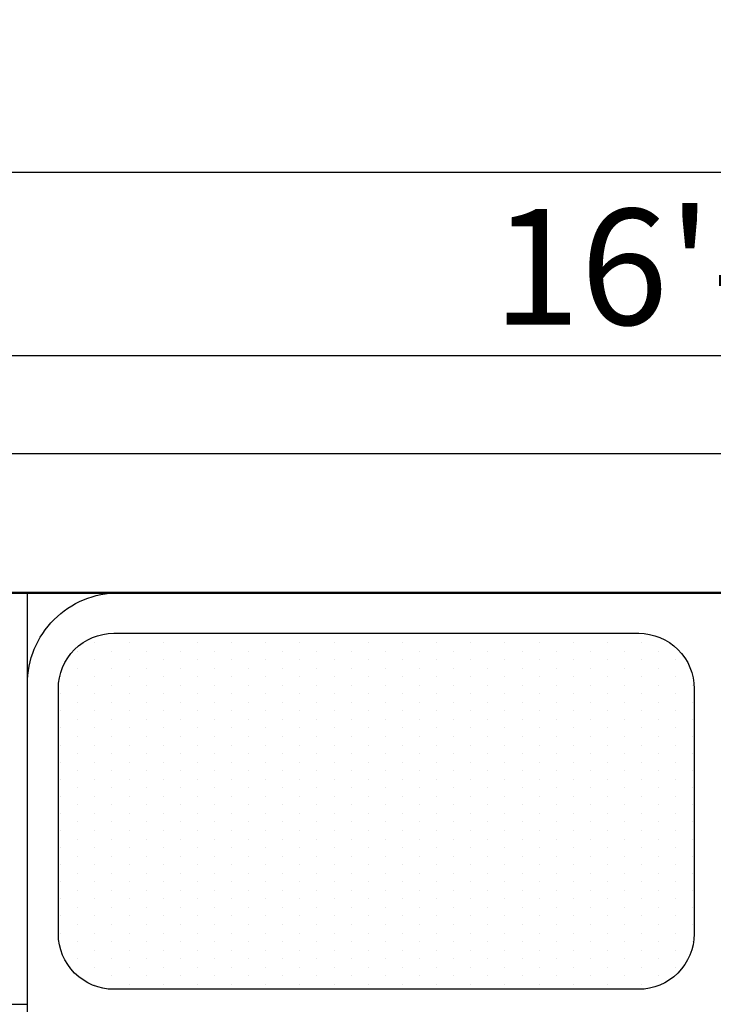
# Model space of a CAD drawing. Units: inches. Extents: x 3064 to 19385, y 846 to 15425.
# Tile 62 of 108: x 6251 to 6281, y 1964 to 2007. Entities that reach past the tile are written whole.
import ezdxf

# ---------------------------------------------------------------- set-up
doc = ezdxf.new("R2010")
doc.units = ezdxf.units.IN
for name, color, linetype, lineweight in [('A-ANNO-DIMS', 2, 'Continuous', 18), ('A-FLOR-FIXT', 9, 'Continuous', 18), ('A-WALL', 7, 'Continuous', 50), ('C-PROP', 6, 'Continuous', 25)]:
    doc.layers.add(name, color=color, linetype=linetype, lineweight=lineweight)
doc.layers.add('BLOCK', color=6, linetype='Continuous')
doc.styles.get("Standard").update_dxf_attribs({"font": 'arial.ttf'})
doc.dimstyles.new('ISO-25', dxfattribs={"dimtxt": 9, "dimasz": 2.5, "dimexe": 1.25, "dimexo": 0.625, "dimtad": 1, "dimdec": 1, "dimlunit": 3, "dimtxsty": 'Standard', "dimcen": 2.5, "dimadec": 0, "dimazin": 0, "dimtfac": 1, "dimtdec": 1, "dimtmove": 0, "dimatfit": 3, "dimfxl": 1, "dimarcsym": 0})

# ---------------------------------------------------------------- blocks, each defined once
blk = doc.blocks.new('*X7')
at = {"color": 0}
for p, q in [((266.25, 456.9375), (266.25, 456.9375)), ((266.4375, 457.03125), (266.4375, 457.03125)), ((266.625, 456.9375), (266.625, 456.9375)), ((266.8125, 457.03125), (266.8125, 457.03125)), ((267, 456.9375), (267, 456.9375)), ((267.1875, 457.03125), (267.1875, 457.03125)), ((267.375, 456.9375), (267.375, 456.9375)), ((267.5625, 457.03125), (267.5625, 457.03125)), ((267.75, 456.9375), (267.75, 456.9375)), ((267.9375, 457.03125), (267.9375, 457.03125)), ((268.125, 456.9375), (268.125, 456.9375)), ((268.3125, 457.03125), (268.3125, 457.03125)), ((268.5, 456.9375), (268.5, 456.9375)), ((268.6875, 457.03125), (268.6875, 457.03125)), ((268.875, 456.9375), (268.875, 456.9375)), ((269.0625, 457.03125), (269.0625, 457.03125)), ((269.25, 456.9375), (269.25, 456.9375)), ((269.4375, 457.03125), (269.4375, 457.03125)), ((269.625, 456.9375), (269.625, 456.9375)), ((269.8125, 457.03125), (269.8125, 457.03125)), ((270, 456.9375), (270, 456.9375)), ((270.1875, 457.03125), (270.1875, 457.03125)), ((270.375, 456.9375), (270.375, 456.9375)), ((270.5625, 457.03125), (270.5625, 457.03125)), ((270.75, 456.9375), (270.75, 456.9375)), ((270.9375, 457.03125), (270.9375, 457.03125)), ((271.125, 456.9375), (271.125, 456.9375)), ((271.3125, 457.03125), (271.3125, 457.03125)), ((271.5, 456.9375), (271.5, 456.9375)), ((271.6875, 457.03125), (271.6875, 457.03125)), ((271.875, 456.9375), (271.875, 456.9375)), ((272.0625, 457.03125), (272.0625, 457.03125)), ((272.25, 456.9375), (272.25, 456.9375)), ((266.0625, 456.84375), (266.0625, 456.84375)), ((266.4375, 456.84375), (266.4375, 456.84375)), ((266.8125, 456.84375), (266.8125, 456.84375)), ((267.1875, 456.84375), (267.1875, 456.84375)), ((267.5625, 456.84375), (267.5625, 456.84375)), ((267.9375, 456.84375), (267.9375, 456.84375)), ((268.3125, 456.84375), (268.3125, 456.84375)), ((268.6875, 456.84375), (268.6875, 456.84375)), ((269.0625, 456.84375), (269.0625, 456.84375)), ((269.4375, 456.84375), (269.4375, 456.84375)), ((269.8125, 456.84375), (269.8125, 456.84375)), ((270.1875, 456.84375), (270.1875, 456.84375)), ((270.5625, 456.84375), (270.5625, 456.84375)), ((270.9375, 456.84375), (270.9375, 456.84375)), ((271.3125, 456.84375), (271.3125, 456.84375)), ((271.6875, 456.84375), (271.6875, 456.84375)), ((272.0625, 456.84375), (272.0625, 456.84375)), ((272.4375, 456.84375), (272.4375, 456.84375)), ((266.25, 456.75), (266.25, 456.75)), ((266.625, 456.75), (266.625, 456.75)), ((267, 456.75), (267, 456.75)), ((267.375, 456.75), (267.375, 456.75)), ((267.75, 456.75), (267.75, 456.75)), ((268.125, 456.75), (268.125, 456.75)), ((268.5, 456.75), (268.5, 456.75)), ((268.875, 456.75), (268.875, 456.75)), ((269.25, 456.75), (269.25, 456.75)), ((269.625, 456.75), (269.625, 456.75)), ((270, 456.75), (270, 456.75)), ((270.375, 456.75), (270.375, 456.75)), ((270.75, 456.75), (270.75, 456.75)), ((271.125, 456.75), (271.125, 456.75)), ((271.5, 456.75), (271.5, 456.75)), ((271.875, 456.75), (271.875, 456.75)), ((272.25, 456.75), (272.25, 456.75)), ((272.625, 456.75), (272.625, 456.75)), ((266.0625, 456.65625), (266.0625, 456.65625)), ((266.4375, 456.65625), (266.4375, 456.65625)), ((266.8125, 456.65625), (266.8125, 456.65625)), ((267.1875, 456.65625), (267.1875, 456.65625)), ((267.5625, 456.65625), (267.5625, 456.65625)), ((267.9375, 456.65625), (267.9375, 456.65625)), ((268.3125, 456.65625), (268.3125, 456.65625)), ((268.6875, 456.65625), (268.6875, 456.65625)), ((269.0625, 456.65625), (269.0625, 456.65625)), ((269.4375, 456.65625), (269.4375, 456.65625)), ((269.8125, 456.65625), (269.8125, 456.65625)), ((270.1875, 456.65625), (270.1875, 456.65625)), ((270.5625, 456.65625), (270.5625, 456.65625)), ((270.9375, 456.65625), (270.9375, 456.65625)), ((271.3125, 456.65625), (271.3125, 456.65625)), ((271.6875, 456.65625), (271.6875, 456.65625)), ((272.0625, 456.65625), (272.0625, 456.65625)), ((272.4375, 456.65625), (272.4375, 456.65625)), ((265.875, 456.5625), (265.875, 456.5625)), ((266.25, 456.5625), (266.25, 456.5625)), ((266.625, 456.5625), (266.625, 456.5625)), ((267, 456.5625), (267, 456.5625)), ((267.375, 456.5625), (267.375, 456.5625)), ((267.75, 456.5625), (267.75, 456.5625)), ((268.125, 456.5625), (268.125, 456.5625)), ((268.5, 456.5625), (268.5, 456.5625)), ((268.875, 456.5625), (268.875, 456.5625)), ((269.25, 456.5625), (269.25, 456.5625)), ((269.625, 456.5625), (269.625, 456.5625)), ((270, 456.5625), (270, 456.5625)), ((270.375, 456.5625), (270.375, 456.5625)), ((270.75, 456.5625), (270.75, 456.5625)), ((271.125, 456.5625), (271.125, 456.5625)), ((271.5, 456.5625), (271.5, 456.5625)), ((271.875, 456.5625), (271.875, 456.5625)), ((272.25, 456.5625), (272.25, 456.5625)), ((272.625, 456.5625), (272.625, 456.5625)), ((266.0625, 456.46875), (266.0625, 456.46875)), ((266.4375, 456.46875), (266.4375, 456.46875)), ((266.8125, 456.46875), (266.8125, 456.46875)), ((267.1875, 456.46875), (267.1875, 456.46875)), ((267.5625, 456.46875), (267.5625, 456.46875)), ((267.9375, 456.46875), (267.9375, 456.46875)), ((268.3125, 456.46875), (268.3125, 456.46875)), ((268.6875, 456.46875), (268.6875, 456.46875)), ((269.0625, 456.46875), (269.0625, 456.46875)), ((269.4375, 456.46875), (269.4375, 456.46875)), ((269.8125, 456.46875), (269.8125, 456.46875)), ((270.1875, 456.46875), (270.1875, 456.46875)), ((270.5625, 456.46875), (270.5625, 456.46875)), ((270.9375, 456.46875), (270.9375, 456.46875)), ((271.3125, 456.46875), (271.3125, 456.46875)), ((271.6875, 456.46875), (271.6875, 456.46875)), ((272.0625, 456.46875), (272.0625, 456.46875)), ((272.4375, 456.46875), (272.4375, 456.46875)), ((272.8125, 456.46875), (272.8125, 456.46875)), ((265.875, 456.375), (265.875, 456.375)), ((266.25, 456.375), (266.25, 456.375)), ((266.625, 456.375), (266.625, 456.375)), ((267, 456.375), (267, 456.375)), ((267.375, 456.375), (267.375, 456.375)), ((267.75, 456.375), (267.75, 456.375)), ((268.125, 456.375), (268.125, 456.375)), ((268.5, 456.375), (268.5, 456.375)), ((268.875, 456.375), (268.875, 456.375)), ((269.25, 456.375), (269.25, 456.375)), ((269.625, 456.375), (269.625, 456.375)), ((270, 456.375), (270, 456.375)), ((270.375, 456.375), (270.375, 456.375)), ((270.75, 456.375), (270.75, 456.375)), ((271.125, 456.375), (271.125, 456.375)), ((271.5, 456.375), (271.5, 456.375)), ((271.875, 456.375), (271.875, 456.375)), ((272.25, 456.375), (272.25, 456.375)), ((272.625, 456.375), (272.625, 456.375)), ((265.875, 456.1875), (265.875, 456.1875)), ((266.0625, 456.28125), (266.0625, 456.28125)), ((266.25, 456.1875), (266.25, 456.1875)), ((266.4375, 456.28125), (266.4375, 456.28125)), ((266.625, 456.1875), (266.625, 456.1875)), ((266.8125, 456.28125), (266.8125, 456.28125)), ((267, 456.1875), (267, 456.1875)), ((267.1875, 456.28125), (267.1875, 456.28125)), ((267.375, 456.1875), (267.375, 456.1875)), ((267.5625, 456.28125), (267.5625, 456.28125)), ((267.75, 456.1875), (267.75, 456.1875)), ((267.9375, 456.28125), (267.9375, 456.28125)), ((268.125, 456.1875), (268.125, 456.1875)), ((268.3125, 456.28125), (268.3125, 456.28125)), ((268.5, 456.1875), (268.5, 456.1875)), ((268.6875, 456.28125), (268.6875, 456.28125)), ((268.875, 456.1875), (268.875, 456.1875)), ((269.0625, 456.28125), (269.0625, 456.28125)), ((269.25, 456.1875), (269.25, 456.1875)), ((269.4375, 456.28125), (269.4375, 456.28125)), ((269.625, 456.1875), (269.625, 456.1875)), ((269.8125, 456.28125), (269.8125, 456.28125)), ((270, 456.1875), (270, 456.1875)), ((270.1875, 456.28125), (270.1875, 456.28125)), ((270.375, 456.1875), (270.375, 456.1875)), ((270.5625, 456.28125), (270.5625, 456.28125)), ((270.75, 456.1875), (270.75, 456.1875)), ((270.9375, 456.28125), (270.9375, 456.28125)), ((271.125, 456.1875), (271.125, 456.1875)), ((271.3125, 456.28125), (271.3125, 456.28125)), ((271.5, 456.1875), (271.5, 456.1875)), ((271.6875, 456.28125), (271.6875, 456.28125)), ((271.875, 456.1875), (271.875, 456.1875)), ((272.0625, 456.28125), (272.0625, 456.28125)), ((272.25, 456.1875), (272.25, 456.1875)), ((272.4375, 456.28125), (272.4375, 456.28125)), ((272.625, 456.1875), (272.625, 456.1875)), ((272.8125, 456.28125), (272.8125, 456.28125)), ((266.0625, 456.09375), (266.0625, 456.09375)), ((266.4375, 456.09375), (266.4375, 456.09375)), ((266.8125, 456.09375), (266.8125, 456.09375)), ((267.1875, 456.09375), (267.1875, 456.09375)), ((267.5625, 456.09375), (267.5625, 456.09375)), ((267.9375, 456.09375), (267.9375, 456.09375)), ((268.3125, 456.09375), (268.3125, 456.09375)), ((268.6875, 456.09375), (268.6875, 456.09375)), ((269.0625, 456.09375), (269.0625, 456.09375)), ((269.4375, 456.09375), (269.4375, 456.09375)), ((269.8125, 456.09375), (269.8125, 456.09375)), ((270.1875, 456.09375), (270.1875, 456.09375)), ((270.5625, 456.09375), (270.5625, 456.09375)), ((270.9375, 456.09375), (270.9375, 456.09375)), ((271.3125, 456.09375), (271.3125, 456.09375)), ((271.6875, 456.09375), (271.6875, 456.09375)), ((272.0625, 456.09375), (272.0625, 456.09375)), ((272.4375, 456.09375), (272.4375, 456.09375)), ((272.8125, 456.09375), (272.8125, 456.09375)), ((265.875, 456), (265.875, 456)), ((266.25, 456), (266.25, 456)), ((266.625, 456), (266.625, 456)), ((267, 456), (267, 456)), ((267.375, 456), (267.375, 456)), ((267.75, 456), (267.75, 456)), ((268.125, 456), (268.125, 456)), ((268.5, 456), (268.5, 456)), ((268.875, 456), (268.875, 456)), ((269.25, 456), (269.25, 456)), ((269.625, 456), (269.625, 456)), ((270, 456), (270, 456)), ((270.375, 456), (270.375, 456)), ((270.75, 456), (270.75, 456)), ((271.125, 456), (271.125, 456)), ((271.5, 456), (271.5, 456)), ((271.875, 456), (271.875, 456)), ((272.25, 456), (272.25, 456)), ((272.625, 456), (272.625, 456)), ((266.0625, 455.90625), (266.0625, 455.90625)), ((266.4375, 455.90625), (266.4375, 455.90625)), ((266.8125, 455.90625), (266.8125, 455.90625)), ((267.1875, 455.90625), (267.1875, 455.90625)), ((267.5625, 455.90625), (267.5625, 455.90625)), ((267.9375, 455.90625), (267.9375, 455.90625)), ((268.3125, 455.90625), (268.3125, 455.90625)), ((268.6875, 455.90625), (268.6875, 455.90625)), ((269.0625, 455.90625), (269.0625, 455.90625)), ((269.4375, 455.90625), (269.4375, 455.90625)), ((269.8125, 455.90625), (269.8125, 455.90625)), ((270.1875, 455.90625), (270.1875, 455.90625)), ((270.5625, 455.90625), (270.5625, 455.90625)), ((270.9375, 455.90625), (270.9375, 455.90625)), ((271.3125, 455.90625), (271.3125, 455.90625)), ((271.6875, 455.90625), (271.6875, 455.90625)), ((272.0625, 455.90625), (272.0625, 455.90625)), ((272.4375, 455.90625), (272.4375, 455.90625)), ((272.8125, 455.90625), (272.8125, 455.90625)), ((265.875, 455.8125), (265.875, 455.8125)), ((266.25, 455.8125), (266.25, 455.8125)), ((266.625, 455.8125), (266.625, 455.8125)), ((267, 455.8125), (267, 455.8125)), ((267.375, 455.8125), (267.375, 455.8125)), ((267.75, 455.8125), (267.75, 455.8125)), ((268.125, 455.8125), (268.125, 455.8125)), ((268.5, 455.8125), (268.5, 455.8125)), ((268.875, 455.8125), (268.875, 455.8125)), ((269.25, 455.8125), (269.25, 455.8125)), ((269.625, 455.8125), (269.625, 455.8125)), ((270, 455.8125), (270, 455.8125)), ((270.375, 455.8125), (270.375, 455.8125)), ((270.75, 455.8125), (270.75, 455.8125)), ((271.125, 455.8125), (271.125, 455.8125)), ((271.5, 455.8125), (271.5, 455.8125)), ((271.875, 455.8125), (271.875, 455.8125)), ((272.25, 455.8125), (272.25, 455.8125)), ((272.625, 455.8125), (272.625, 455.8125)), ((266.0625, 455.71875), (266.0625, 455.71875)), ((266.4375, 455.71875), (266.4375, 455.71875)), ((266.8125, 455.71875), (266.8125, 455.71875)), ((267.1875, 455.71875), (267.1875, 455.71875)), ((267.5625, 455.71875), (267.5625, 455.71875)), ((267.9375, 455.71875), (267.9375, 455.71875)), ((268.3125, 455.71875), (268.3125, 455.71875)), ((268.6875, 455.71875), (268.6875, 455.71875)), ((269.0625, 455.71875), (269.0625, 455.71875)), ((269.4375, 455.71875), (269.4375, 455.71875)), ((269.8125, 455.71875), (269.8125, 455.71875)), ((270.1875, 455.71875), (270.1875, 455.71875)), ((270.5625, 455.71875), (270.5625, 455.71875)), ((270.9375, 455.71875), (270.9375, 455.71875)), ((271.3125, 455.71875), (271.3125, 455.71875)), ((271.6875, 455.71875), (271.6875, 455.71875)), ((272.0625, 455.71875), (272.0625, 455.71875)), ((272.4375, 455.71875), (272.4375, 455.71875)), ((272.8125, 455.71875), (272.8125, 455.71875)), ((265.875, 455.625), (265.875, 455.625)), ((266.0625, 455.53125), (266.0625, 455.53125)), ((266.25, 455.625), (266.25, 455.625)), ((266.4375, 455.53125), (266.4375, 455.53125)), ((266.625, 455.625), (266.625, 455.625)), ((266.8125, 455.53125), (266.8125, 455.53125)), ((267, 455.625), (267, 455.625)), ((267.1875, 455.53125), (267.1875, 455.53125)), ((267.375, 455.625), (267.375, 455.625)), ((267.5625, 455.53125), (267.5625, 455.53125)), ((267.75, 455.625), (267.75, 455.625)), ((267.9375, 455.53125), (267.9375, 455.53125)), ((268.125, 455.625), (268.125, 455.625)), ((268.3125, 455.53125), (268.3125, 455.53125)), ((268.5, 455.625), (268.5, 455.625)), ((268.6875, 455.53125), (268.6875, 455.53125)), ((268.875, 455.625), (268.875, 455.625)), ((269.0625, 455.53125), (269.0625, 455.53125)), ((269.25, 455.625), (269.25, 455.625)), ((269.4375, 455.53125), (269.4375, 455.53125)), ((269.625, 455.625), (269.625, 455.625)), ((269.8125, 455.53125), (269.8125, 455.53125)), ((270, 455.625), (270, 455.625)), ((270.1875, 455.53125), (270.1875, 455.53125)), ((270.375, 455.625), (270.375, 455.625)), ((270.5625, 455.53125), (270.5625, 455.53125)), ((270.75, 455.625), (270.75, 455.625)), ((270.9375, 455.53125), (270.9375, 455.53125)), ((271.125, 455.625), (271.125, 455.625)), ((271.3125, 455.53125), (271.3125, 455.53125)), ((271.5, 455.625), (271.5, 455.625)), ((271.6875, 455.53125), (271.6875, 455.53125)), ((271.875, 455.625), (271.875, 455.625)), ((272.0625, 455.53125), (272.0625, 455.53125)), ((272.25, 455.625), (272.25, 455.625)), ((272.4375, 455.53125), (272.4375, 455.53125)), ((272.625, 455.625), (272.625, 455.625)), ((272.8125, 455.53125), (272.8125, 455.53125)), ((265.875, 455.4375), (265.875, 455.4375)), ((266.25, 455.4375), (266.25, 455.4375)), ((266.625, 455.4375), (266.625, 455.4375)), ((267, 455.4375), (267, 455.4375)), ((267.375, 455.4375), (267.375, 455.4375)), ((267.75, 455.4375), (267.75, 455.4375)), ((268.125, 455.4375), (268.125, 455.4375)), ((268.5, 455.4375), (268.5, 455.4375)), ((268.875, 455.4375), (268.875, 455.4375)), ((269.25, 455.4375), (269.25, 455.4375)), ((269.625, 455.4375), (269.625, 455.4375)), ((270, 455.4375), (270, 455.4375)), ((270.375, 455.4375), (270.375, 455.4375)), ((270.75, 455.4375), (270.75, 455.4375)), ((271.125, 455.4375), (271.125, 455.4375)), ((271.5, 455.4375), (271.5, 455.4375)), ((271.875, 455.4375), (271.875, 455.4375)), ((272.25, 455.4375), (272.25, 455.4375)), ((272.625, 455.4375), (272.625, 455.4375)), ((266.0625, 455.34375), (266.0625, 455.34375)), ((266.4375, 455.34375), (266.4375, 455.34375)), ((266.8125, 455.34375), (266.8125, 455.34375)), ((267.1875, 455.34375), (267.1875, 455.34375)), ((267.5625, 455.34375), (267.5625, 455.34375)), ((267.9375, 455.34375), (267.9375, 455.34375)), ((268.3125, 455.34375), (268.3125, 455.34375)), ((268.6875, 455.34375), (268.6875, 455.34375)), ((269.0625, 455.34375), (269.0625, 455.34375)), ((269.4375, 455.34375), (269.4375, 455.34375)), ((269.8125, 455.34375), (269.8125, 455.34375)), ((270.1875, 455.34375), (270.1875, 455.34375)), ((270.5625, 455.34375), (270.5625, 455.34375)), ((270.9375, 455.34375), (270.9375, 455.34375)), ((271.3125, 455.34375), (271.3125, 455.34375)), ((271.6875, 455.34375), (271.6875, 455.34375)), ((272.0625, 455.34375), (272.0625, 455.34375)), ((272.4375, 455.34375), (272.4375, 455.34375)), ((272.8125, 455.34375), (272.8125, 455.34375)), ((265.875, 455.25), (265.875, 455.25)), ((266.25, 455.25), (266.25, 455.25)), ((266.625, 455.25), (266.625, 455.25)), ((267, 455.25), (267, 455.25)), ((267.375, 455.25), (267.375, 455.25)), ((267.75, 455.25), (267.75, 455.25)), ((268.125, 455.25), (268.125, 455.25)), ((268.5, 455.25), (268.5, 455.25)), ((268.875, 455.25), (268.875, 455.25)), ((269.25, 455.25), (269.25, 455.25)), ((269.625, 455.25), (269.625, 455.25)), ((270, 455.25), (270, 455.25)), ((270.375, 455.25), (270.375, 455.25)), ((270.75, 455.25), (270.75, 455.25)), ((271.125, 455.25), (271.125, 455.25)), ((271.5, 455.25), (271.5, 455.25)), ((271.875, 455.25), (271.875, 455.25)), ((272.25, 455.25), (272.25, 455.25)), ((272.625, 455.25), (272.625, 455.25)), ((266.0625, 455.15625), (266.0625, 455.15625)), ((266.4375, 455.15625), (266.4375, 455.15625)), ((266.8125, 455.15625), (266.8125, 455.15625)), ((267.1875, 455.15625), (267.1875, 455.15625)), ((267.5625, 455.15625), (267.5625, 455.15625)), ((267.9375, 455.15625), (267.9375, 455.15625)), ((268.3125, 455.15625), (268.3125, 455.15625)), ((268.6875, 455.15625), (268.6875, 455.15625)), ((269.0625, 455.15625), (269.0625, 455.15625)), ((269.4375, 455.15625), (269.4375, 455.15625)), ((269.8125, 455.15625), (269.8125, 455.15625)), ((270.1875, 455.15625), (270.1875, 455.15625)), ((270.5625, 455.15625), (270.5625, 455.15625)), ((270.9375, 455.15625), (270.9375, 455.15625)), ((271.3125, 455.15625), (271.3125, 455.15625)), ((271.6875, 455.15625), (271.6875, 455.15625)), ((272.0625, 455.15625), (272.0625, 455.15625)), ((272.4375, 455.15625), (272.4375, 455.15625)), ((272.8125, 455.15625), (272.8125, 455.15625)), ((265.875, 455.0625), (265.875, 455.0625)), ((266.25, 455.0625), (266.25, 455.0625)), ((266.625, 455.0625), (266.625, 455.0625)), ((267, 455.0625), (267, 455.0625)), ((267.375, 455.0625), (267.375, 455.0625)), ((267.75, 455.0625), (267.75, 455.0625)), ((268.125, 455.0625), (268.125, 455.0625)), ((268.5, 455.0625), (268.5, 455.0625)), ((268.875, 455.0625), (268.875, 455.0625)), ((269.25, 455.0625), (269.25, 455.0625)), ((269.625, 455.0625), (269.625, 455.0625)), ((270, 455.0625), (270, 455.0625)), ((270.375, 455.0625), (270.375, 455.0625)), ((270.75, 455.0625), (270.75, 455.0625)), ((271.125, 455.0625), (271.125, 455.0625)), ((271.5, 455.0625), (271.5, 455.0625)), ((271.875, 455.0625), (271.875, 455.0625)), ((272.25, 455.0625), (272.25, 455.0625)), ((272.625, 455.0625), (272.625, 455.0625)), ((266.0625, 454.96875), (266.0625, 454.96875)), ((266.4375, 454.96875), (266.4375, 454.96875)), ((266.8125, 454.96875), (266.8125, 454.96875)), ((267.1875, 454.96875), (267.1875, 454.96875)), ((267.5625, 454.96875), (267.5625, 454.96875)), ((267.9375, 454.96875), (267.9375, 454.96875)), ((268.3125, 454.96875), (268.3125, 454.96875)), ((268.6875, 454.96875), (268.6875, 454.96875)), ((269.0625, 454.96875), (269.0625, 454.96875)), ((269.4375, 454.96875), (269.4375, 454.96875)), ((269.8125, 454.96875), (269.8125, 454.96875)), ((270.1875, 454.96875), (270.1875, 454.96875)), ((270.5625, 454.96875), (270.5625, 454.96875)), ((270.9375, 454.96875), (270.9375, 454.96875)), ((271.3125, 454.96875), (271.3125, 454.96875)), ((271.6875, 454.96875), (271.6875, 454.96875)), ((272.0625, 454.96875), (272.0625, 454.96875)), ((272.4375, 454.96875), (272.4375, 454.96875)), ((272.8125, 454.96875), (272.8125, 454.96875)), ((265.875, 454.875), (265.875, 454.875)), ((266.0625, 454.78125), (266.0625, 454.78125)), ((266.25, 454.875), (266.25, 454.875)), ((266.4375, 454.78125), (266.4375, 454.78125)), ((266.625, 454.875), (266.625, 454.875)), ((266.8125, 454.78125), (266.8125, 454.78125)), ((267, 454.875), (267, 454.875)), ((267.1875, 454.78125), (267.1875, 454.78125)), ((267.375, 454.875), (267.375, 454.875)), ((267.5625, 454.78125), (267.5625, 454.78125)), ((267.75, 454.875), (267.75, 454.875)), ((267.9375, 454.78125), (267.9375, 454.78125)), ((268.125, 454.875), (268.125, 454.875)), ((268.3125, 454.78125), (268.3125, 454.78125)), ((268.5, 454.875), (268.5, 454.875)), ((268.6875, 454.78125), (268.6875, 454.78125)), ((268.875, 454.875), (268.875, 454.875)), ((269.0625, 454.78125), (269.0625, 454.78125)), ((269.25, 454.875), (269.25, 454.875)), ((269.4375, 454.78125), (269.4375, 454.78125)), ((269.625, 454.875), (269.625, 454.875)), ((269.8125, 454.78125), (269.8125, 454.78125)), ((270, 454.875), (270, 454.875)), ((270.1875, 454.78125), (270.1875, 454.78125)), ((270.375, 454.875), (270.375, 454.875)), ((270.5625, 454.78125), (270.5625, 454.78125)), ((270.75, 454.875), (270.75, 454.875)), ((270.9375, 454.78125), (270.9375, 454.78125)), ((271.125, 454.875), (271.125, 454.875)), ((271.3125, 454.78125), (271.3125, 454.78125)), ((271.5, 454.875), (271.5, 454.875)), ((271.6875, 454.78125), (271.6875, 454.78125)), ((271.875, 454.875), (271.875, 454.875)), ((272.0625, 454.78125), (272.0625, 454.78125)), ((272.25, 454.875), (272.25, 454.875)), ((272.4375, 454.78125), (272.4375, 454.78125)), ((272.625, 454.875), (272.625, 454.875)), ((272.8125, 454.78125), (272.8125, 454.78125)), ((265.875, 454.6875), (265.875, 454.6875)), ((266.25, 454.6875), (266.25, 454.6875)), ((266.625, 454.6875), (266.625, 454.6875)), ((267, 454.6875), (267, 454.6875)), ((267.375, 454.6875), (267.375, 454.6875)), ((267.75, 454.6875), (267.75, 454.6875)), ((268.125, 454.6875), (268.125, 454.6875)), ((268.5, 454.6875), (268.5, 454.6875)), ((268.875, 454.6875), (268.875, 454.6875)), ((269.25, 454.6875), (269.25, 454.6875)), ((269.625, 454.6875), (269.625, 454.6875)), ((270, 454.6875), (270, 454.6875)), ((270.375, 454.6875), (270.375, 454.6875)), ((270.75, 454.6875), (270.75, 454.6875)), ((271.125, 454.6875), (271.125, 454.6875)), ((271.5, 454.6875), (271.5, 454.6875)), ((271.875, 454.6875), (271.875, 454.6875)), ((272.25, 454.6875), (272.25, 454.6875)), ((272.625, 454.6875), (272.625, 454.6875)), ((266.0625, 454.59375), (266.0625, 454.59375)), ((266.4375, 454.59375), (266.4375, 454.59375)), ((266.8125, 454.59375), (266.8125, 454.59375)), ((267.1875, 454.59375), (267.1875, 454.59375)), ((267.5625, 454.59375), (267.5625, 454.59375)), ((267.9375, 454.59375), (267.9375, 454.59375)), ((268.3125, 454.59375), (268.3125, 454.59375)), ((268.6875, 454.59375), (268.6875, 454.59375)), ((269.0625, 454.59375), (269.0625, 454.59375)), ((269.4375, 454.59375), (269.4375, 454.59375)), ((269.8125, 454.59375), (269.8125, 454.59375)), ((270.1875, 454.59375), (270.1875, 454.59375)), ((270.5625, 454.59375), (270.5625, 454.59375)), ((270.9375, 454.59375), (270.9375, 454.59375)), ((271.3125, 454.59375), (271.3125, 454.59375)), ((271.6875, 454.59375), (271.6875, 454.59375)), ((272.0625, 454.59375), (272.0625, 454.59375)), ((272.4375, 454.59375), (272.4375, 454.59375)), ((272.8125, 454.59375), (272.8125, 454.59375)), ((265.875, 454.5), (265.875, 454.5)), ((266.25, 454.5), (266.25, 454.5)), ((266.625, 454.5), (266.625, 454.5)), ((267, 454.5), (267, 454.5)), ((267.375, 454.5), (267.375, 454.5)), ((267.75, 454.5), (267.75, 454.5)), ((268.125, 454.5), (268.125, 454.5)), ((268.5, 454.5), (268.5, 454.5)), ((268.875, 454.5), (268.875, 454.5)), ((269.25, 454.5), (269.25, 454.5)), ((269.625, 454.5), (269.625, 454.5)), ((270, 454.5), (270, 454.5)), ((270.375, 454.5), (270.375, 454.5)), ((270.75, 454.5), (270.75, 454.5)), ((271.125, 454.5), (271.125, 454.5)), ((271.5, 454.5), (271.5, 454.5)), ((271.875, 454.5), (271.875, 454.5)), ((272.25, 454.5), (272.25, 454.5)), ((272.625, 454.5), (272.625, 454.5)), ((266.0625, 454.40625), (266.0625, 454.40625)), ((266.4375, 454.40625), (266.4375, 454.40625)), ((266.8125, 454.40625), (266.8125, 454.40625)), ((267.1875, 454.40625), (267.1875, 454.40625)), ((267.5625, 454.40625), (267.5625, 454.40625)), ((267.9375, 454.40625), (267.9375, 454.40625)), ((268.3125, 454.40625), (268.3125, 454.40625)), ((268.6875, 454.40625), (268.6875, 454.40625)), ((269.0625, 454.40625), (269.0625, 454.40625)), ((269.4375, 454.40625), (269.4375, 454.40625)), ((269.8125, 454.40625), (269.8125, 454.40625)), ((270.1875, 454.40625), (270.1875, 454.40625)), ((270.5625, 454.40625), (270.5625, 454.40625)), ((270.9375, 454.40625), (270.9375, 454.40625)), ((271.3125, 454.40625), (271.3125, 454.40625)), ((271.6875, 454.40625), (271.6875, 454.40625)), ((272.0625, 454.40625), (272.0625, 454.40625)), ((272.4375, 454.40625), (272.4375, 454.40625)), ((272.8125, 454.40625), (272.8125, 454.40625)), ((265.875, 454.3125), (265.875, 454.3125)), ((266.25, 454.3125), (266.25, 454.3125)), ((266.625, 454.3125), (266.625, 454.3125)), ((267, 454.3125), (267, 454.3125)), ((267.375, 454.3125), (267.375, 454.3125)), ((267.75, 454.3125), (267.75, 454.3125)), ((268.125, 454.3125), (268.125, 454.3125)), ((268.5, 454.3125), (268.5, 454.3125)), ((268.875, 454.3125), (268.875, 454.3125)), ((269.25, 454.3125), (269.25, 454.3125)), ((269.625, 454.3125), (269.625, 454.3125)), ((270, 454.3125), (270, 454.3125)), ((270.375, 454.3125), (270.375, 454.3125)), ((270.75, 454.3125), (270.75, 454.3125)), ((271.125, 454.3125), (271.125, 454.3125)), ((271.5, 454.3125), (271.5, 454.3125)), ((271.875, 454.3125), (271.875, 454.3125)), ((272.25, 454.3125), (272.25, 454.3125)), ((272.625, 454.3125), (272.625, 454.3125)), ((266.0625, 454.21875), (266.0625, 454.21875)), ((266.4375, 454.21875), (266.4375, 454.21875)), ((266.8125, 454.21875), (266.8125, 454.21875)), ((267.1875, 454.21875), (267.1875, 454.21875)), ((267.5625, 454.21875), (267.5625, 454.21875)), ((267.9375, 454.21875), (267.9375, 454.21875)), ((268.3125, 454.21875), (268.3125, 454.21875)), ((268.6875, 454.21875), (268.6875, 454.21875)), ((269.0625, 454.21875), (269.0625, 454.21875)), ((269.4375, 454.21875), (269.4375, 454.21875)), ((269.8125, 454.21875), (269.8125, 454.21875)), ((270.1875, 454.21875), (270.1875, 454.21875)), ((270.5625, 454.21875), (270.5625, 454.21875)), ((270.9375, 454.21875), (270.9375, 454.21875)), ((271.3125, 454.21875), (271.3125, 454.21875)), ((271.6875, 454.21875), (271.6875, 454.21875)), ((272.0625, 454.21875), (272.0625, 454.21875)), ((272.4375, 454.21875), (272.4375, 454.21875)), ((272.8125, 454.21875), (272.8125, 454.21875)), ((265.875, 454.125), (265.875, 454.125)), ((266.0625, 454.03125), (266.0625, 454.03125)), ((266.25, 454.125), (266.25, 454.125)), ((266.4375, 454.03125), (266.4375, 454.03125)), ((266.625, 454.125), (266.625, 454.125)), ((266.8125, 454.03125), (266.8125, 454.03125)), ((267, 454.125), (267, 454.125)), ((267.1875, 454.03125), (267.1875, 454.03125)), ((267.375, 454.125), (267.375, 454.125)), ((267.5625, 454.03125), (267.5625, 454.03125)), ((267.75, 454.125), (267.75, 454.125)), ((267.9375, 454.03125), (267.9375, 454.03125)), ((268.125, 454.125), (268.125, 454.125)), ((268.3125, 454.03125), (268.3125, 454.03125)), ((268.5, 454.125), (268.5, 454.125)), ((268.6875, 454.03125), (268.6875, 454.03125)), ((268.875, 454.125), (268.875, 454.125)), ((269.0625, 454.03125), (269.0625, 454.03125)), ((269.25, 454.125), (269.25, 454.125)), ((269.4375, 454.03125), (269.4375, 454.03125)), ((269.625, 454.125), (269.625, 454.125)), ((269.8125, 454.03125), (269.8125, 454.03125)), ((270, 454.125), (270, 454.125)), ((270.1875, 454.03125), (270.1875, 454.03125)), ((270.375, 454.125), (270.375, 454.125)), ((270.5625, 454.03125), (270.5625, 454.03125)), ((270.75, 454.125), (270.75, 454.125)), ((270.9375, 454.03125), (270.9375, 454.03125)), ((271.125, 454.125), (271.125, 454.125)), ((271.3125, 454.03125), (271.3125, 454.03125)), ((271.5, 454.125), (271.5, 454.125)), ((271.6875, 454.03125), (271.6875, 454.03125)), ((271.875, 454.125), (271.875, 454.125)), ((272.0625, 454.03125), (272.0625, 454.03125)), ((272.25, 454.125), (272.25, 454.125)), ((272.4375, 454.03125), (272.4375, 454.03125)), ((272.625, 454.125), (272.625, 454.125)), ((272.8125, 454.03125), (272.8125, 454.03125)), ((265.875, 453.9375), (265.875, 453.9375)), ((266.25, 453.9375), (266.25, 453.9375)), ((266.625, 453.9375), (266.625, 453.9375)), ((267, 453.9375), (267, 453.9375)), ((267.375, 453.9375), (267.375, 453.9375)), ((267.75, 453.9375), (267.75, 453.9375)), ((268.125, 453.9375), (268.125, 453.9375)), ((268.5, 453.9375), (268.5, 453.9375)), ((268.875, 453.9375), (268.875, 453.9375)), ((269.25, 453.9375), (269.25, 453.9375)), ((269.625, 453.9375), (269.625, 453.9375)), ((270, 453.9375), (270, 453.9375)), ((270.375, 453.9375), (270.375, 453.9375)), ((270.75, 453.9375), (270.75, 453.9375)), ((271.125, 453.9375), (271.125, 453.9375)), ((271.5, 453.9375), (271.5, 453.9375)), ((271.875, 453.9375), (271.875, 453.9375)), ((272.25, 453.9375), (272.25, 453.9375)), ((272.625, 453.9375), (272.625, 453.9375)), ((266.0625, 453.84375), (266.0625, 453.84375)), ((266.4375, 453.84375), (266.4375, 453.84375)), ((266.8125, 453.84375), (266.8125, 453.84375)), ((267.1875, 453.84375), (267.1875, 453.84375)), ((267.5625, 453.84375), (267.5625, 453.84375)), ((267.9375, 453.84375), (267.9375, 453.84375)), ((268.3125, 453.84375), (268.3125, 453.84375)), ((268.6875, 453.84375), (268.6875, 453.84375)), ((269.0625, 453.84375), (269.0625, 453.84375)), ((269.4375, 453.84375), (269.4375, 453.84375)), ((269.8125, 453.84375), (269.8125, 453.84375)), ((270.1875, 453.84375), (270.1875, 453.84375)), ((270.5625, 453.84375), (270.5625, 453.84375)), ((270.9375, 453.84375), (270.9375, 453.84375)), ((271.3125, 453.84375), (271.3125, 453.84375)), ((271.6875, 453.84375), (271.6875, 453.84375)), ((272.0625, 453.84375), (272.0625, 453.84375)), ((272.4375, 453.84375), (272.4375, 453.84375)), ((272.8125, 453.84375), (272.8125, 453.84375)), ((265.875, 453.75), (265.875, 453.75)), ((266.25, 453.75), (266.25, 453.75)), ((266.625, 453.75), (266.625, 453.75)), ((267, 453.75), (267, 453.75)), ((267.375, 453.75), (267.375, 453.75)), ((267.75, 453.75), (267.75, 453.75)), ((268.125, 453.75), (268.125, 453.75)), ((268.5, 453.75), (268.5, 453.75)), ((268.875, 453.75), (268.875, 453.75)), ((269.25, 453.75), (269.25, 453.75)), ((269.625, 453.75), (269.625, 453.75)), ((270, 453.75), (270, 453.75)), ((270.375, 453.75), (270.375, 453.75)), ((270.75, 453.75), (270.75, 453.75)), ((271.125, 453.75), (271.125, 453.75)), ((271.5, 453.75), (271.5, 453.75)), ((271.875, 453.75), (271.875, 453.75)), ((272.25, 453.75), (272.25, 453.75)), ((272.625, 453.75), (272.625, 453.75)), ((266.0625, 453.65625), (266.0625, 453.65625)), ((266.4375, 453.65625), (266.4375, 453.65625)), ((266.8125, 453.65625), (266.8125, 453.65625)), ((267.1875, 453.65625), (267.1875, 453.65625)), ((267.5625, 453.65625), (267.5625, 453.65625)), ((267.9375, 453.65625), (267.9375, 453.65625)), ((268.3125, 453.65625), (268.3125, 453.65625)), ((268.6875, 453.65625), (268.6875, 453.65625)), ((269.0625, 453.65625), (269.0625, 453.65625)), ((269.4375, 453.65625), (269.4375, 453.65625)), ((269.8125, 453.65625), (269.8125, 453.65625)), ((270.1875, 453.65625), (270.1875, 453.65625)), ((270.5625, 453.65625), (270.5625, 453.65625)), ((270.9375, 453.65625), (270.9375, 453.65625)), ((271.3125, 453.65625), (271.3125, 453.65625)), ((271.6875, 453.65625), (271.6875, 453.65625)), ((272.0625, 453.65625), (272.0625, 453.65625)), ((272.4375, 453.65625), (272.4375, 453.65625)), ((272.8125, 453.65625), (272.8125, 453.65625)), ((266.25, 453.5625), (266.25, 453.5625)), ((266.625, 453.5625), (266.625, 453.5625)), ((267, 453.5625), (267, 453.5625)), ((267.375, 453.5625), (267.375, 453.5625)), ((267.75, 453.5625), (267.75, 453.5625)), ((268.125, 453.5625), (268.125, 453.5625)), ((268.5, 453.5625), (268.5, 453.5625)), ((268.875, 453.5625), (268.875, 453.5625)), ((269.25, 453.5625), (269.25, 453.5625)), ((269.625, 453.5625), (269.625, 453.5625)), ((270, 453.5625), (270, 453.5625)), ((270.375, 453.5625), (270.375, 453.5625)), ((270.75, 453.5625), (270.75, 453.5625)), ((271.125, 453.5625), (271.125, 453.5625)), ((271.5, 453.5625), (271.5, 453.5625)), ((271.875, 453.5625), (271.875, 453.5625)), ((272.25, 453.5625), (272.25, 453.5625)), ((272.625, 453.5625), (272.625, 453.5625)), ((266.0625, 453.46875), (266.0625, 453.46875)), ((266.25, 453.375), (266.25, 453.375)), ((266.4375, 453.46875), (266.4375, 453.46875)), ((266.625, 453.375), (266.625, 453.375)), ((266.8125, 453.46875), (266.8125, 453.46875)), ((267, 453.375), (267, 453.375)), ((267.1875, 453.46875), (267.1875, 453.46875)), ((267.375, 453.375), (267.375, 453.375)), ((267.5625, 453.46875), (267.5625, 453.46875)), ((267.75, 453.375), (267.75, 453.375)), ((267.9375, 453.46875), (267.9375, 453.46875)), ((268.125, 453.375), (268.125, 453.375)), ((268.3125, 453.46875), (268.3125, 453.46875)), ((268.5, 453.375), (268.5, 453.375)), ((268.6875, 453.46875), (268.6875, 453.46875)), ((268.875, 453.375), (268.875, 453.375)), ((269.0625, 453.46875), (269.0625, 453.46875)), ((269.25, 453.375), (269.25, 453.375)), ((269.4375, 453.46875), (269.4375, 453.46875)), ((269.625, 453.375), (269.625, 453.375)), ((269.8125, 453.46875), (269.8125, 453.46875)), ((270, 453.375), (270, 453.375)), ((270.1875, 453.46875), (270.1875, 453.46875)), ((270.375, 453.375), (270.375, 453.375)), ((270.5625, 453.46875), (270.5625, 453.46875)), ((270.75, 453.375), (270.75, 453.375)), ((270.9375, 453.46875), (270.9375, 453.46875)), ((271.125, 453.375), (271.125, 453.375)), ((271.3125, 453.46875), (271.3125, 453.46875)), ((271.5, 453.375), (271.5, 453.375)), ((271.6875, 453.46875), (271.6875, 453.46875)), ((271.875, 453.375), (271.875, 453.375)), ((272.0625, 453.46875), (272.0625, 453.46875)), ((272.25, 453.375), (272.25, 453.375)), ((272.4375, 453.46875), (272.4375, 453.46875)), ((272.625, 453.375), (272.625, 453.375)), ((266.0625, 453.28125), (266.0625, 453.28125)), ((266.4375, 453.28125), (266.4375, 453.28125)), ((266.8125, 453.28125), (266.8125, 453.28125)), ((267.1875, 453.28125), (267.1875, 453.28125)), ((267.5625, 453.28125), (267.5625, 453.28125)), ((267.9375, 453.28125), (267.9375, 453.28125)), ((268.3125, 453.28125), (268.3125, 453.28125)), ((268.6875, 453.28125), (268.6875, 453.28125)), ((269.0625, 453.28125), (269.0625, 453.28125)), ((269.4375, 453.28125), (269.4375, 453.28125)), ((269.8125, 453.28125), (269.8125, 453.28125)), ((270.1875, 453.28125), (270.1875, 453.28125)), ((270.5625, 453.28125), (270.5625, 453.28125)), ((270.9375, 453.28125), (270.9375, 453.28125)), ((271.3125, 453.28125), (271.3125, 453.28125)), ((271.6875, 453.28125), (271.6875, 453.28125)), ((272.0625, 453.28125), (272.0625, 453.28125)), ((272.4375, 453.28125), (272.4375, 453.28125)), ((266.25, 453.1875), (266.25, 453.1875)), ((266.625, 453.1875), (266.625, 453.1875)), ((267, 453.1875), (267, 453.1875)), ((267.375, 453.1875), (267.375, 453.1875)), ((267.75, 453.1875), (267.75, 453.1875)), ((268.125, 453.1875), (268.125, 453.1875)), ((268.5, 453.1875), (268.5, 453.1875)), ((268.875, 453.1875), (268.875, 453.1875)), ((269.25, 453.1875), (269.25, 453.1875)), ((269.625, 453.1875), (269.625, 453.1875)), ((270, 453.1875), (270, 453.1875)), ((270.375, 453.1875), (270.375, 453.1875)), ((270.75, 453.1875), (270.75, 453.1875)), ((271.125, 453.1875), (271.125, 453.1875)), ((271.5, 453.1875), (271.5, 453.1875)), ((271.875, 453.1875), (271.875, 453.1875)), ((272.25, 453.1875), (272.25, 453.1875))]:
    blk.add_line(p, q, dxfattribs=at)
blk = doc.blocks.new('A$C52E67D0D')
at = {"layer": 'BLOCK'}
blk.add_lwpolyline([(501, 1348.6), (501, 1799.6), (0, 1799.6), (0, 1348.6)], close=True, dxfattribs=at)
for points in [[(1901, 0), (601, 0, -0.414214), (501, 100), (501, 1700, -0.414214), (601, 1800), (1901, 1800, -0.414214), (2001, 1700), (2001, 100, -0.414214)], [(1171.8, 1365.1), (595.8, 1365.1, -0.414214), (535, 1425.9), (535, 1694.8, -0.414214), (595.8, 1755.7), (1171.8, 1755.7, -0.414214), (1232.6, 1694.8), (1232.6, 1425.9, -0.414214)]]:
    blk.add_lwpolyline(points, format="xyb", close=True, dxfattribs=at)
blk.add_arc((1888.6, -1664.5), 3015.3, 87.8642, 117.4001, dxfattribs=at)
at = {"layer": 'BLOCK', "xscale": 100, "yscale": 100, "zscale": 100}
blk.add_blockref('*X7', (-26050, -43948.2), dxfattribs=at)
blk = doc.blocks.new('*D387')
at = {"layer": 'A-ANNO-DIMS', "color": 0, "lineweight": -2, "transparency": 16777216}
for p, q in [((6183.493, 1988.614), (6183.493, 1993.494)), ((6378.493, 1988.614), (6378.493, 1993.494)), ((6185.993, 1992.244), (6375.993, 1992.244))]:
    blk.add_line(p, q, dxfattribs=at)
at = {"layer": 'A-ANNO-DIMS', "color": 0, "transparency": 16777216}
for points in [[(6185.993, 1992.66), (6185.993, 1991.827), (6183.493, 1992.244)], [(6375.993, 1992.66), (6375.993, 1991.827), (6378.493, 1992.244)]]:
    blk.add_solid(points, dxfattribs=at)
at = {"layer": 'Defpoints', "color": 0, "transparency": 16777216}
for p in [(6378.493, 1992.244), (6183.493, 1987.989), (6378.493, 1987.989)]:
    blk.add_point(p, dxfattribs=at)
at = {"layer": 'A-ANNO-DIMS', "color": 0, "transparency": 16777216, "insert": (6280.993, 1995.423), "char_height": 5, "attachment_point": 5}
blk.add_mtext('16\'-3"', dxfattribs=at)
blk = doc.blocks.new('*D378')
at = {"layer": 'A-ANNO-DIMS', "color": 0, "lineweight": -2, "transparency": 16777216}
for p, q in [((6042.493, 1988.614), (6042.493, 2001.412)), ((6384.493, 1988.614), (6384.493, 2001.412)), ((6044.993, 2000.162), (6381.993, 2000.162))]:
    blk.add_line(p, q, dxfattribs=at)
at = {"layer": 'A-ANNO-DIMS', "color": 0, "transparency": 16777216}
for points in [[(6044.993, 2000.578), (6044.993, 1999.745), (6042.493, 2000.162)], [(6381.993, 2000.578), (6381.993, 1999.745), (6384.493, 2000.162)]]:
    blk.add_solid(points, dxfattribs=at)
at = {"layer": 'Defpoints', "color": 0, "transparency": 16777216}
for p in [(6384.493, 2000.162), (6042.493, 1987.989), (6384.493, 1987.989)]:
    blk.add_point(p, dxfattribs=at)
at = {"layer": 'A-ANNO-DIMS', "color": 0, "transparency": 16777216, "insert": (6213.493, 2003.34), "char_height": 5, "attachment_point": 5}
blk.add_mtext('28\'-6"', dxfattribs=at)

msp = doc.modelspace()

# ---------------------------------------------------------------- linework, layer by layer
at = {"layer": 'A-WALL'}
msp.add_line((6378.493, 1981.989), (6183.493, 1981.989), dxfattribs=at)
at = {"layer": 'C-PROP'}
msp.add_line((6384.493, 1987.989), (6042.493, 1987.989), dxfattribs=at)

# ---------------------------------------------------------------- block references
at = {"layer": 'A-FLOR-FIXT', "xscale": 0.039370099999992, "yscale": 0.039370099999992, "zscale": 0.039370099999992}
msp.add_blockref('A$C52E67D0D', (6231.741, 1911.123), dxfattribs=at)

# ---------------------------------------------------------------- dimensions: what is measured, and where the dimension line sits
at = {"layer": 'A-ANNO-DIMS'}
for base, p1, p2, override, picture, middle in [((6384.493, 2000.162), (6042.493, 1987.989), (6384.493, 1987.989), {"dimtxt": 5, "dimclrd": 0, "dimclre": 0, "dimclrt": 0}, '*D378', (6213.493, 2003.34)), ((6378.493, 1992.244), (6183.493, 1987.989), (6378.493, 1987.989), {"dimtxt": 5, "dimclrd": 0, "dimclre": 0, "dimclrt": 0, "dimtmove": 1}, '*D387', (6280.993, 1995.423))]:
    dim = msp.add_linear_dim(base=base, p1=p1, p2=p2, dimstyle='ISO-25', override=override, dxfattribs=at)
    dim.commit()
    dim.dimension.update_dxf_attribs({"geometry": picture, "text_midpoint": middle})

doc.saveas('drawing.dxf')
